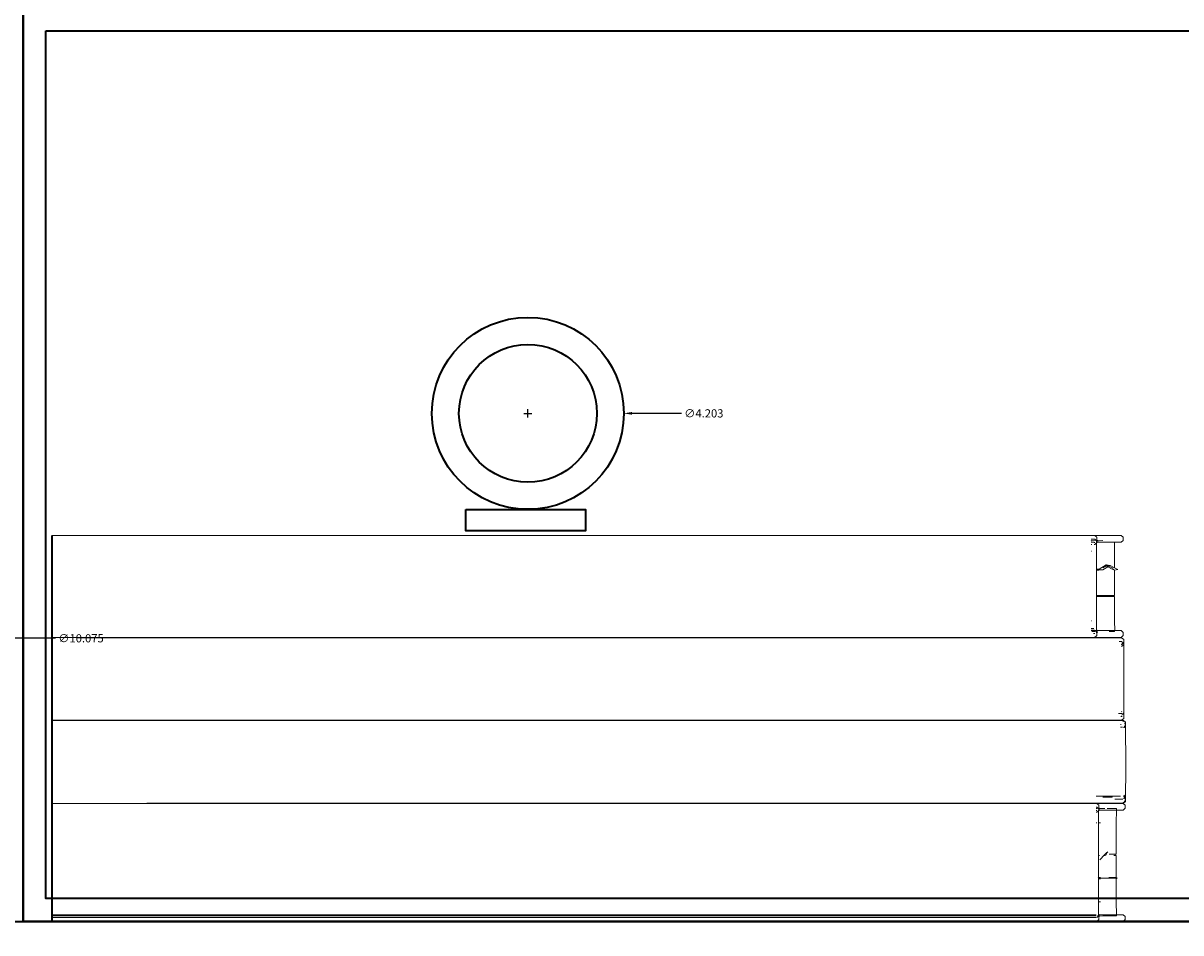
# Model space of a CAD drawing. Units: millimetres. Extents: x 446512 to 447461, y 70395 to 70610.
# Tile 17 of 39: x 446699 to 446725, y 70493 to 70513. Entities that reach past the tile are written whole.
import ezdxf

# ---------------------------------------------------------------- set-up
doc = ezdxf.new("R2010")
doc.units = ezdxf.units.MM
for name, color, linetype, lineweight in [('A-ANNO-DIMS', 2, 'Continuous', 18), ('A-FURN', 7, 'Continuous', 35), ('A-FURN-DECO', 8, 'Continuous', 13)]:
    doc.layers.add(name, color=color, linetype=linetype, lineweight=lineweight)
doc.styles.get("Standard").update_dxf_attribs({"font": 'arial.ttf'})
doc.dimstyles.get("Standard").update_dxf_attribs({"dimtxt": 0.18, "dimasz": 0.18, "dimexe": 0.18, "dimexo": 0.0625, "dimgap": 0.09, "dimtad": 0, "dimtih": 1, "dimtoh": 1, "dimdec": 4, "dimzin": 0, "dimdsep": 46, "dimtxsty": 'Standard', "dimcen": 0.09, "dimadec": 0, "dimazin": 0, "dimtfac": 1, "dimtdec": 4, "dimtofl": 0, "dimtmove": 0, "dimatfit": 3, "dimfxl": 1, "dimtolj": 1, "dimtzin": 0, "dimarcsym": 0})

# ---------------------------------------------------------------- blocks, each defined once
blk = doc.blocks.new('*D75')
at = {"layer": 'A-ANNO-DIMS', "color": 0, "lineweight": -2, "transparency": 16777216}
for p, q in [((446691.984, 70499.581), (446692.164, 70499.581)), ((446692.074, 70499.491), (446692.074, 70499.671)), ((446700.134, 70499.581), (446697.291, 70499.581))]:
    blk.add_line(p, q, dxfattribs=at)
at = {"layer": 'A-ANNO-DIMS', "color": 0, "transparency": 16777216}
blk.add_solid([(446697.291, 70499.611), (446697.291, 70499.551), (446697.111, 70499.581)], dxfattribs=at)
at = {"layer": 'Defpoints', "color": 0, "transparency": 16777216}
for p in [(446687.036, 70499.58), (446697.111, 70499.581)]:
    blk.add_point(p, dxfattribs=at)
at = {"layer": 'A-ANNO-DIMS', "color": 0, "transparency": 16777216, "insert": (446700.696, 70499.581), "char_height": 0.18, "attachment_point": 5}
blk.add_mtext('\\A1;∅10.075', dxfattribs=at)
blk = doc.blocks.new('*D77')
at = {"layer": 'A-ANNO-DIMS', "color": 0, "lineweight": -2, "transparency": 16777216}
for p, q in [((446710.394, 70504.505), (446710.574, 70504.505)), ((446710.484, 70504.415), (446710.484, 70504.595)), ((446713.847, 70504.505), (446712.766, 70504.505))]:
    blk.add_line(p, q, dxfattribs=at)
at = {"layer": 'A-ANNO-DIMS', "color": 0, "transparency": 16777216}
blk.add_solid([(446712.766, 70504.535), (446712.766, 70504.475), (446712.586, 70504.505)], dxfattribs=at)
at = {"layer": 'Defpoints', "color": 0, "transparency": 16777216}
for p in [(446708.383, 70504.506), (446712.586, 70504.505)]:
    blk.add_point(p, dxfattribs=at)
at = {"layer": 'A-ANNO-DIMS', "color": 0, "transparency": 16777216, "insert": (446714.338, 70504.505), "char_height": 0.18, "attachment_point": 5}
blk.add_mtext('\\A1;∅4.203', dxfattribs=at)

msp = doc.modelspace()

# ---------------------------------------------------------------- linework, layer by layer
at = {"layer": 'A-FURN'}
for p, q in [((446699.4288, 70513.3815), (446699.4288, 70493.3815)), ((446700.0643, 70493.3815), (446700.0643, 70501.8335)), ((446686.5728, 70493.3815), (446746.5728, 70493.3815))]:
    msp.add_line(p, q, dxfattribs=at)
for points in [[(446699.4288, 70513.3815), (446746.5728, 70513.3815), (446746.5728, 70493.3815), (446699.4288, 70493.3815)], [(446699.9288, 70512.8815), (446746.0728, 70512.8815), (446746.0728, 70493.8815), (446699.9288, 70493.8815)], [(446709.124, 70502.4015), (446711.7437, 70502.4015), (446711.7437, 70501.9339), (446709.124, 70501.9339)], [(446686.5728, 70493.3815), (446729.0084, 70493.3815), (446729.0084, 70473.3815), (446686.5728, 70473.3815)]]:
    msp.add_lwpolyline(points, close=True, dxfattribs=at)
for radius in [2.1014, 1.509]:
    msp.add_circle((446710.4845, 70504.5054), radius, dxfattribs=at)
at = {"layer": 'A-FURN-DECO'}
for p, q in [((446722.8971, 70501.8335), (446700.0643, 70501.8335)), ((446722.9157, 70501.8176), (446722.8971, 70501.8335)), ((446723.4803, 70501.8335), (446722.8971, 70501.8335)), ((446723.4803, 70501.8335), (446723.5262, 70501.7912)), ((446722.8352, 70501.6354), (446722.8233, 70501.6354)), ((446722.8288, 70501.7172), (446722.8234, 70501.7189)), ((446722.8234, 70501.6823), (446722.8913, 70501.6823)), ((446722.9054, 70501.7478), (446722.8235, 70501.7478)), ((446722.9205, 70501.7189), (446722.8288, 70501.7172)), ((446722.8982, 70501.676), (446722.8913, 70501.676)), ((446722.9054, 70501.6354), (446722.8913, 70501.6354)), ((446722.9015, 70501.6784), (446722.8982, 70501.676)), ((446722.9274, 70501.7275), (446722.9054, 70501.7478)), ((446722.9415, 70501.6688), (446722.9054, 70501.6354)), ((446722.9157, 70501.8176), (446722.9407, 70501.7992)), ((446722.9385, 70501.7172), (446722.9429, 70501.7175)), ((446722.943, 70501.713), (446722.9385, 70501.7172)), ((446722.9431, 70501.7102), (446722.9385, 70501.7067)), ((446722.9385, 70501.6823), (446722.9431, 70501.7102)), ((446722.9416, 70501.6777), (446722.9385, 70501.6823)), ((446722.9418, 70501.6823), (446722.9385, 70501.6823)), ((446722.9408, 70501.796), (446722.9407, 70501.7992)), ((446722.9435, 70501.7937), (446722.9408, 70501.796)), ((446722.941, 70501.4147), (446722.9413, 70501.6291)), ((446722.9413, 70501.6291), (446722.9415, 70501.6688)), ((446722.9512, 70501.6778), (446722.9415, 70501.6688)), ((446722.9415, 70501.6688), (446722.9416, 70501.6777)), ((446722.9525, 70501.6797), (446722.9418, 70501.6823)), ((446722.9429, 70501.7175), (446722.9461, 70501.7595)), ((446722.9429, 70501.7175), (446722.9499, 70501.7194)), ((446722.943, 70501.713), (446722.9429, 70501.7175)), ((446722.9512, 70501.7055), (446722.943, 70501.713)), ((446722.9431, 70501.7102), (446722.943, 70501.713)), ((446722.9461, 70501.7595), (446722.9435, 70501.7937)), ((446722.9499, 70501.7194), (446722.9461, 70501.7595)), ((446722.959, 70501.7246), (446722.9499, 70501.7194)), ((446722.9499, 70501.7194), (446722.9575, 70501.7183)), ((446722.9512, 70501.7055), (446722.9499, 70501.7194)), ((446722.9512, 70501.6778), (446722.9525, 70501.6797)), ((446722.9525, 70501.6797), (446722.9537, 70501.6907)), ((446722.9525, 70501.6797), (446722.9689, 70501.6823)), ((446722.9537, 70501.6907), (446722.9563, 70501.7131)), ((446722.9563, 70501.7131), (446722.9575, 70501.7183)), ((446722.9575, 70501.7183), (446722.959, 70501.7246)), ((446722.9575, 70501.7183), (446722.9672, 70501.7189)), ((446722.9689, 70501.6823), (446723.3347, 70501.6823)), ((446722.9919, 70501.7178), (446722.9821, 70501.7189)), ((446723.0764, 70501.7189), (446722.9919, 70501.7178)), ((446723.3347, 70501.6823), (446723.3328, 70501.4843)), ((446723.3347, 70501.6823), (446723.4803, 70501.6823)), ((446723.5262, 70501.7246), (446723.4803, 70501.6823)), ((446723.5262, 70501.7912), (446723.5262, 70501.7246)), ((446722.8269, 70501.4843), (446722.8232, 70501.4843)), ((446722.9383, 70501.0962), (446722.941, 70501.4147)), ((446723.3328, 70501.4843), (446723.3311, 70501.2268)), ((446722.9382, 70501.0737), (446722.9383, 70501.081)), ((446722.9382, 70501.0737), (446722.9408, 70501.0705)), ((446722.9382, 70501.0705), (446722.9382, 70501.0737)), ((446722.9408, 70501.0705), (446722.9382, 70501.0705)), ((446722.9407, 70500.9576), (446722.9382, 70501.0705)), ((446722.9408, 70501.0931), (446722.9383, 70501.0962)), ((446722.9383, 70501.0931), (446722.9383, 70501.0962)), ((446722.9383, 70501.0931), (446722.9408, 70501.0931)), ((446722.9383, 70501.0849), (446722.9383, 70501.0931)), ((446722.9383, 70501.0849), (446722.9408, 70501.0849)), ((446722.9383, 70501.081), (446722.9383, 70501.0849)), ((446722.9383, 70501.081), (446723.0064, 70501.0816)), ((446722.9845, 70501.0962), (446722.9408, 70501.0931)), ((446722.9408, 70501.0849), (446723.0064, 70501.0816)), ((446722.9879, 70501.0709), (446722.9408, 70501.0705)), ((446722.9845, 70501.0962), (446722.9879, 70501.0935)), ((446722.9879, 70501.0935), (446722.9926, 70501.0962)), ((446722.9927, 70501.0737), (446722.9879, 70501.0709)), ((446722.9962, 70501.0962), (446722.9926, 70501.0962)), ((446723.0795, 70501.0822), (446722.9927, 70501.0737)), ((446723.0064, 70501.0816), (446722.9927, 70501.0737)), ((446722.9962, 70501.0962), (446723.1508, 70501.1872)), ((446723.0064, 70501.0816), (446723.0093, 70501.0849)), ((446723.0795, 70501.0822), (446723.0093, 70501.0849)), ((446723.1507, 70501.1646), (446723.0776, 70501.1225)), ((446723.0795, 70501.0822), (446723.189, 70501.1452)), ((446723.1867, 70501.169), (446723.1507, 70501.1646)), ((446723.1729, 70501.1534), (446723.1507, 70501.1646)), ((446723.2423, 70501.1759), (446723.1508, 70501.1872)), ((446723.1508, 70501.1872), (446723.1867, 70501.169)), ((446723.2423, 70501.1759), (446723.1867, 70501.169)), ((446723.1867, 70501.169), (446723.2001, 70501.1622)), ((446723.189, 70501.1452), (446723.2099, 70501.1572)), ((446723.2861, 70501.0962), (446723.189, 70501.1452)), ((446723.2099, 70501.1572), (446723.2423, 70501.1759)), ((446723.2099, 70501.1572), (446723.296, 70501.1137)), ((446723.3308, 70501.126), (446723.2423, 70501.1759)), ((446723.3112, 70501.0962), (446723.2861, 70501.0962)), ((446723.3084, 70501.0849), (446723.2861, 70501.0962)), ((446723.3084, 70501.0849), (446723.3209, 70501.0849)), ((446723.3306, 70501.0737), (446723.3084, 70501.0849)), ((446723.3306, 70501.0737), (446723.3302, 70500.9431)), ((446723.4036, 70501.0849), (446723.3306, 70501.0737)), ((446723.3311, 70501.2268), (446723.3308, 70501.126)), ((446723.4036, 70501.0849), (446723.3308, 70501.126)), ((446722.9382, 70500.515), (446722.9407, 70500.9576)), ((446723.3302, 70500.515), (446723.3302, 70500.9431)), ((446722.9382, 70500.515), (446722.9875, 70500.5152)), ((446722.9382, 70500.4925), (446722.9382, 70500.515)), ((446722.9407, 70500.4471), (446722.9382, 70500.4925)), ((446722.9407, 70500.4925), (446722.9382, 70500.4925)), ((446722.9407, 70500.4925), (446722.9875, 70500.4926)), ((446722.9407, 70500.4471), (446722.9413, 70499.8035)), ((446722.9875, 70500.5152), (446723.3302, 70500.515)), ((446722.9875, 70500.4926), (446723.3303, 70500.4925)), ((446723.3302, 70500.515), (446723.1845, 70500.5038)), ((446723.1845, 70500.5038), (446723.3303, 70500.4925)), ((446723.3311, 70500.22), (446723.3303, 70500.4925)), ((446723.3311, 70500.22), (446723.3328, 70499.9625)), ((446722.8232, 70499.9625), (446722.8269, 70499.9625)), ((446722.9415, 70499.764), (446722.9413, 70499.8035)), ((446723.3328, 70499.9625), (446723.3382, 70499.7505)), ((446722.8971, 70499.5993), (446700.0643, 70499.5993)), ((446723.4896, 70499.5923), (446700.6021, 70499.5923)), ((446722.8794, 70499.7974), (446722.8233, 70499.7974)), ((446722.8924, 70499.7568), (446722.8234, 70499.7568)), ((446722.8234, 70499.7505), (446722.9065, 70499.7505)), ((446722.8402, 70499.7296), (446722.9199, 70499.7279)), ((446722.9199, 70499.7279), (446722.8415, 70499.7279)), ((446722.9002, 70499.685), (446722.876, 70499.685)), ((446722.8971, 70499.5993), (446722.9407, 70499.6336)), ((446722.8971, 70499.5993), (446723.4803, 70499.5993)), ((446722.9065, 70499.7505), (446722.9015, 70499.7543)), ((446722.9131, 70499.7505), (446722.9065, 70499.7505)), ((446722.9131, 70499.7505), (446722.9252, 70499.7394)), ((446722.9241, 70499.737), (446722.9131, 70499.7505)), ((446722.9303, 70499.7505), (446722.9131, 70499.7505)), ((446722.9415, 70499.764), (446722.9372, 70499.768)), ((446722.9385, 70499.7505), (446722.9416, 70499.7551)), ((446722.9418, 70499.7505), (446722.9385, 70499.7505)), ((446722.9385, 70499.7292), (446722.9385, 70499.7505)), ((446722.9385, 70499.7292), (446722.9429, 70499.7271)), ((446722.9429, 70499.7271), (446722.9385, 70499.727)), ((446722.943, 70499.7198), (446722.9385, 70499.7156)), ((446722.9407, 70499.6336), (446722.9436, 70499.6383)), ((446722.9416, 70499.7551), (446722.9415, 70499.764)), ((446722.9512, 70499.755), (446722.9415, 70499.764)), ((446722.9525, 70499.7531), (446722.9418, 70499.7505)), ((446722.9512, 70499.7273), (446722.9429, 70499.7271)), ((446722.9431, 70499.7225), (446722.9429, 70499.7271)), ((446722.9431, 70499.7225), (446722.943, 70499.7198)), ((446722.943, 70499.7198), (446722.9461, 70499.6702)), ((446722.943, 70499.7198), (446722.9499, 70499.7144)), ((446722.9512, 70499.7273), (446722.9431, 70499.7225)), ((446722.9436, 70499.6383), (446722.9461, 70499.6702)), ((446722.9461, 70499.6702), (446722.9499, 70499.7144)), ((446722.9499, 70499.7144), (446722.9512, 70499.7273)), ((446722.9499, 70499.7144), (446722.959, 70499.7081)), ((446722.9525, 70499.7531), (446722.9512, 70499.755)), ((446722.9689, 70499.7505), (446722.9525, 70499.7531)), ((446722.9538, 70499.7414), (446722.9525, 70499.7531)), ((446722.9563, 70499.7197), (446722.9538, 70499.7414)), ((446722.959, 70499.7081), (446722.9563, 70499.7197)), ((446723.3382, 70499.7505), (446722.9689, 70499.7505)), ((446723.2189, 70499.7283), (446723.2219, 70499.7279)), ((446723.335, 70499.7279), (446723.2219, 70499.7279)), ((446723.3382, 70499.7505), (446723.335, 70499.7279)), ((446723.3382, 70499.7505), (446723.4803, 70499.7505)), ((446723.4803, 70499.7505), (446723.5262, 70499.7081)), ((446723.5262, 70499.6416), (446723.4803, 70499.5993)), ((446723.4896, 70499.5923), (446723.5354, 70499.5511)), ((446723.5354, 70499.5535), (446723.4896, 70499.5923)), ((446723.4896, 70499.5923), (446723.5354, 70499.5589)), ((446723.5262, 70499.7081), (446723.5262, 70499.6416)), ((446723.5354, 70499.5535), (446723.5354, 70499.5589)), ((446723.5354, 70499.5511), (446723.5354, 70499.5535)), ((446723.5354, 70499.4881), (446723.5354, 70499.5511)), ((446723.4896, 70499.5089), (446723.437, 70499.5089)), ((446723.5241, 70499.4775), (446723.4896, 70499.5089)), ((446723.5241, 70499.4775), (446723.4896, 70499.4452)), ((446723.5327, 70499.4697), (446723.4896, 70499.439)), ((446723.5354, 70499.4407), (446723.4896, 70499.3996)), ((446723.5354, 70499.4881), (446723.5241, 70499.4775)), ((446723.5327, 70499.4697), (446723.5241, 70499.4775)), ((446723.5327, 70499.4697), (446723.5354, 70499.4751)), ((446723.5354, 70499.4717), (446723.5327, 70499.4697)), ((446723.5354, 70499.4673), (446723.5327, 70499.4697)), ((446723.5354, 70499.4751), (446723.5354, 70499.4881)), ((446723.5354, 70499.4751), (446723.5354, 70499.4717)), ((446723.5354, 70499.4717), (446723.5354, 70499.4673)), ((446723.5354, 70499.4695), (446723.5354, 70499.4717)), ((446723.5354, 70499.4673), (446723.5354, 70499.4695)), ((446723.5354, 70499.4407), (446723.5354, 70499.4673)), ((446723.5354, 70499.4407), (446723.5354, 70497.821)), ((446723.4896, 70497.7877), (446700.0643, 70497.7877)), ((446700.0643, 70497.7788), (446723.5109, 70497.7788)), ((446723.4216, 70497.9348), (446723.4896, 70497.9348)), ((446723.4896, 70497.871), (446723.4742, 70497.871)), ((446723.4971, 70497.9736), (446723.4896, 70497.9804)), ((446723.4896, 70497.9348), (446723.5163, 70497.9107)), ((446723.5042, 70497.8841), (446723.4896, 70497.871)), ((446723.5354, 70497.821), (446723.4896, 70497.7877)), ((446723.52, 70497.9188), (446723.4951, 70497.9369)), ((446723.5109, 70497.7788), (446723.5308, 70497.7608)), ((446723.5301, 70497.7788), (446723.5109, 70497.7788)), ((446723.5312, 70497.943), (446723.5252, 70497.9484)), ((446723.5301, 70497.7788), (446723.575, 70497.7454)), ((446723.4802, 70497.6954), (446723.4648, 70497.6954)), ((446723.5109, 70497.6317), (446723.4651, 70497.6317)), ((446723.5374, 70497.6299), (446723.5339, 70497.6313)), ((446723.5374, 70497.6299), (446723.5644, 70497.6542)), ((446723.5631, 70497.657), (446723.5561, 70497.6617)), ((446723.5574, 70497.7324), (446723.5593, 70497.7192)), ((446723.5644, 70497.6272), (446723.5583, 70497.6217)), ((446723.5593, 70497.7192), (446723.5605, 70497.6984)), ((446723.5623, 70497.6697), (446723.5631, 70497.657)), ((446723.5631, 70497.657), (446723.5644, 70497.6542)), ((446723.5644, 70497.6542), (446723.5694, 70497.6538)), ((446723.5658, 70497.6347), (446723.5644, 70497.6272)), ((446723.5694, 70497.6538), (446723.5658, 70497.6347)), ((446723.571, 70497.6582), (446723.5694, 70497.6538)), ((446723.571, 70497.6582), (446723.5732, 70497.684)), ((446723.5734, 70497.6912), (446723.575, 70497.7454)), ((446723.575, 70497.7454), (446723.5772, 70497.6891)), ((446723.5772, 70497.6891), (446723.5782, 70497.4065)), ((446723.5782, 70497.4065), (446723.5788, 70497.0652)), ((446723.5788, 70497.0652), (446723.5788, 70496.6735)), ((446723.5788, 70496.6735), (446723.5776, 70496.1388)), ((446723.2862, 70496.1212), (446722.9288, 70496.1212)), ((446723.2861, 70496.0998), (446723.0748, 70496.0988)), ((446723.2862, 70496.1212), (446723.2861, 70496.0998)), ((446723.4653, 70496.1212), (446723.2862, 70496.1212)), ((446723.5173, 70496.0575), (446723.3433, 70496.0575)), ((446723.575, 70496.0075), (446723.5301, 70495.9741)), ((446723.5631, 70496.0959), (446723.5328, 70496.0703)), ((446723.5644, 70496.0987), (446723.5329, 70496.1223)), ((446723.5644, 70496.1257), (446723.5385, 70496.149)), ((446723.5567, 70496.0153), (446723.5473, 70496.0069)), ((446723.5585, 70496.0282), (446723.5567, 70496.0153)), ((446723.5619, 70496.0757), (446723.5605, 70496.0545)), ((446723.5631, 70496.0959), (446723.5619, 70496.0757)), ((446723.5644, 70496.0987), (446723.5631, 70496.0959)), ((446723.5644, 70496.1257), (446723.5657, 70496.1183)), ((446723.5707, 70496.0978), (446723.5644, 70496.0987)), ((446723.5657, 70496.1183), (446723.5691, 70496.1025)), ((446723.5691, 70496.1025), (446723.5707, 70496.0978)), ((446723.5707, 70496.0978), (446723.5725, 70496.0941)), ((446723.5725, 70496.0941), (446723.5734, 70496.0617)), ((446723.5772, 70496.0638), (446723.5734, 70496.0617)), ((446723.575, 70496.0075), (446723.5734, 70496.0617)), ((446723.5776, 70496.1388), (446723.5772, 70496.0638)), ((446700.0643, 70495.9661), (446722.9411, 70495.9661)), ((446723.5301, 70495.9741), (446702.1377, 70495.9741)), ((446722.9493, 70495.7734), (446722.9349, 70495.7734)), ((446722.9422, 70495.8129), (446722.935, 70495.8129)), ((446722.9618, 70495.8516), (446722.9352, 70495.8515)), ((446722.9494, 70495.8828), (446722.9353, 70495.8828)), ((446722.9596, 70495.9506), (446722.9411, 70495.9661)), ((446722.9411, 70495.9661), (446723.5243, 70495.9661)), ((446722.9453, 70495.8152), (446722.9422, 70495.8129)), ((446722.9854, 70495.8059), (446722.9493, 70495.7734)), ((446722.9713, 70495.863), (446722.9494, 70495.8828)), ((446722.9825, 70495.9315), (446722.9596, 70495.9506)), ((446722.9596, 70495.9506), (446722.9846, 70495.9328)), ((446722.9816, 70495.5392), (446722.9851, 70495.7673)), ((446722.987, 70495.8462), (446722.9823, 70495.8427)), ((446722.9823, 70495.819), (446722.987, 70495.8462)), ((446722.9855, 70495.8145), (446722.9823, 70495.819)), ((446722.9857, 70495.819), (446722.9823, 70495.819)), ((446722.987, 70495.8489), (446722.9824, 70495.8531)), ((446722.9869, 70495.8531), (446722.9824, 70495.8531)), ((446722.9845, 70495.9298), (446722.9846, 70495.9328)), ((446722.9874, 70495.9274), (446722.9845, 70495.9298)), ((446722.9874, 70495.9274), (446722.9846, 70495.9328)), ((446722.9851, 70495.7673), (446722.9854, 70495.8059)), ((446722.9952, 70495.8146), (446722.9854, 70495.8059)), ((446722.9854, 70495.8059), (446722.9855, 70495.8145)), ((446722.9964, 70495.8165), (446722.9857, 70495.819)), ((446722.9869, 70495.8531), (446722.9901, 70495.8941)), ((446722.9938, 70495.8551), (446722.9869, 70495.8531)), ((446722.9869, 70495.8531), (446722.987, 70495.8489)), ((446722.9952, 70495.8416), (446722.987, 70495.8489)), ((446722.987, 70495.8462), (446722.987, 70495.8489)), ((446722.9901, 70495.8941), (446722.9874, 70495.9274)), ((446722.9938, 70495.8551), (446722.9901, 70495.8941)), ((446723.0029, 70495.8602), (446722.9938, 70495.8551)), ((446723.0012, 70495.8531), (446722.9938, 70495.8551)), ((446722.9952, 70495.8416), (446722.9938, 70495.8551)), ((446722.9952, 70495.8146), (446722.9964, 70495.8165)), ((446722.9964, 70495.8165), (446722.9976, 70495.8272)), ((446723.0807, 70495.819), (446722.9964, 70495.8165)), ((446722.9976, 70495.8272), (446723.0003, 70495.849)), ((446723.0003, 70495.849), (446723.0012, 70495.8531)), ((446723.0012, 70495.8531), (446723.0029, 70495.8602)), ((446723.0316, 70495.8518), (446723.0012, 70495.8531)), ((446723.1184, 70495.8529), (446723.0316, 70495.8518)), ((446723.3745, 70495.819), (446723.0807, 70495.819)), ((446723.1721, 70495.8529), (446723.1759, 70495.8523)), ((446723.3747, 70495.8529), (446723.1759, 70495.8523)), ((446723.3745, 70495.819), (446723.3725, 70495.5392)), ((446723.3747, 70495.8529), (446723.3745, 70495.819)), ((446723.3745, 70495.819), (446723.5243, 70495.819)), ((446723.5308, 70495.9921), (446723.5209, 70495.9832)), ((446723.5243, 70495.9661), (446723.5701, 70495.925)), ((446723.5701, 70495.8602), (446723.5243, 70495.819)), ((446723.5701, 70495.925), (446723.5701, 70495.8602)), ((446722.946, 70495.5392), (446722.9342, 70495.5392)), ((446722.9839, 70495.4518), (446722.9816, 70495.5392)), ((446723.0252, 70495.5392), (446722.9816, 70495.5392)), ((446723.3725, 70495.5392), (446723.3708, 70495.2072)), ((446722.9833, 70494.9427), (446722.9839, 70495.4518)), ((446723.37, 70494.8559), (446723.3708, 70495.2072)), ((446722.9808, 70494.8559), (446722.9833, 70494.9427)), ((446722.9808, 70494.8269), (446722.9808, 70494.8559)), ((446722.9808, 70494.8559), (446722.9914, 70494.8559)), ((446722.9833, 70494.3585), (446722.9808, 70494.8269)), ((446723.0026, 70494.8269), (446722.9808, 70494.8269)), ((446723.0114, 70494.7332), (446723.0272, 70494.7478)), ((446723.1026, 70494.8269), (446723.0272, 70494.7478)), ((446723.1026, 70494.8269), (446723.0924, 70494.8269)), ((446723.1372, 70494.8559), (446723.1026, 70494.8269)), ((446723.1026, 70494.8269), (446723.131, 70494.8559)), ((446723.138, 70494.8269), (446723.1139, 70494.8269)), ((446723.1221, 70494.8559), (446723.131, 70494.8559)), ((446723.131, 70494.8559), (446723.1663, 70494.8922)), ((446723.19, 70494.9068), (446723.1372, 70494.8559)), ((446723.1372, 70494.8559), (446723.1677, 70494.8559)), ((446723.1525, 70494.8269), (446723.1489, 70494.8269)), ((446723.19, 70494.9068), (446723.1663, 70494.8922)), ((446723.2167, 70494.8559), (446723.37, 70494.8559)), ((446723.3699, 70494.8269), (446723.3196, 70494.8269)), ((446723.37, 70494.8559), (446723.3383, 70494.8414)), ((446723.3383, 70494.8414), (446723.3699, 70494.8269)), ((446723.3699, 70494.5094), (446723.3699, 70494.8269)), ((446723.3699, 70494.5094), (446723.3703, 70494.341)), ((446722.9791, 70494.341), (446722.9833, 70494.3585)), ((446722.9808, 70494.3265), (446722.9791, 70494.341)), ((446723.0276, 70494.341), (446722.9791, 70494.341)), ((446722.9809, 70494.312), (446722.9808, 70494.3265)), ((446723.3909, 70494.3265), (446722.9808, 70494.3265)), ((446722.9839, 70493.8856), (446722.9809, 70494.312)), ((446722.9809, 70494.312), (446723.0242, 70494.312)), ((446723.3703, 70494.341), (446723.2129, 70494.341)), ((446723.3703, 70494.341), (446723.3909, 70494.3265)), ((446723.3704, 70494.312), (446723.3909, 70494.3265)), ((446723.3708, 70494.1436), (446723.3704, 70494.312)), ((446723.3708, 70494.1436), (446723.3725, 70493.8116)), ((446722.9816, 70493.8116), (446722.9839, 70493.8856)), ((446722.9851, 70493.5802), (446722.9816, 70493.8116)), ((446722.9816, 70493.8116), (446723.0251, 70493.8116)), ((446723.3725, 70493.8116), (446723.3746, 70493.5286)), ((446722.6925, 70493.5286), (446700.0643, 70493.5286)), ((446722.6925, 70493.5071), (446700.0643, 70493.5049)), ((446722.9353, 70493.4649), (446700.0643, 70493.4649)), ((446722.6925, 70493.5286), (446722.6925, 70493.5071)), ((446722.935, 70493.5286), (446722.6925, 70493.5286)), ((446722.6925, 70493.5071), (446722.8685, 70493.5066)), ((446722.8685, 70493.5066), (446722.9351, 70493.505)), ((446722.9494, 70493.4649), (446722.9441, 70493.4649)), ((446722.987, 70493.5015), (446722.9494, 70493.4649)), ((446722.9629, 70493.505), (446722.9834, 70493.505)), ((446722.9834, 70493.505), (446722.9679, 70493.5157)), ((446722.969, 70493.5179), (446722.9834, 70493.505)), ((446722.9857, 70493.5286), (446722.974, 70493.5286)), ((446722.9854, 70493.5418), (446722.9818, 70493.5451)), ((446722.9834, 70493.505), (446722.9857, 70493.5286)), ((446722.987, 70493.5015), (446722.9834, 70493.505)), ((446722.9854, 70493.5418), (446722.9851, 70493.5802)), ((446722.9855, 70493.5331), (446722.9854, 70493.5418)), ((446722.9952, 70493.5331), (446722.9854, 70493.5418)), ((446722.9857, 70493.5286), (446722.9855, 70493.5331)), ((446722.9964, 70493.5311), (446722.9857, 70493.5286)), ((446722.9952, 70493.5061), (446722.987, 70493.5015)), ((446722.987, 70493.5015), (446722.987, 70493.4988)), ((446722.987, 70493.5015), (446722.9939, 70493.4935)), ((446723.0003, 70493.4987), (446722.987, 70493.5015)), ((446722.987, 70493.4988), (446722.99, 70493.4506)), ((446722.99, 70493.4506), (446722.9939, 70493.4935)), ((446722.9939, 70493.4935), (446722.9952, 70493.5061)), ((446722.9939, 70493.4935), (446723.0029, 70493.4875)), ((446722.9964, 70493.5311), (446722.9952, 70493.5331)), ((446722.9952, 70493.5061), (446722.9995, 70493.505)), ((446723.0807, 70493.5286), (446722.9964, 70493.5311)), ((446722.9977, 70493.5199), (446722.9964, 70493.5311)), ((446722.9995, 70493.505), (446722.9977, 70493.5199)), ((446722.9995, 70493.505), (446723.0316, 70493.506)), ((446723.0003, 70493.4987), (446722.9995, 70493.505)), ((446723.1945, 70493.5055), (446723.0003, 70493.4987)), ((446723.0029, 70493.4875), (446723.0003, 70493.4987)), ((446723.0316, 70493.506), (446723.1945, 70493.5055)), ((446723.0807, 70493.5286), (446723.3746, 70493.5286)), ((446723.1945, 70493.5055), (446723.3747, 70493.505)), ((446723.3746, 70493.5286), (446723.3747, 70493.505)), ((446723.3746, 70493.5286), (446723.5243, 70493.5286)), ((446723.5243, 70493.5286), (446723.5701, 70493.4875)), ((446723.5701, 70493.4875), (446723.5701, 70493.4227)), ((446722.9411, 70493.3815), (446700.0643, 70493.3815)), ((446722.9411, 70493.3815), (446722.9846, 70493.4149)), ((446722.9411, 70493.3815), (446723.5243, 70493.3815)), ((446722.9846, 70493.4149), (446722.9875, 70493.4195)), ((446722.9875, 70493.4195), (446722.99, 70493.4506)), ((446723.5701, 70493.4227), (446723.5243, 70493.3815))]:
    msp.add_line(p, q, dxfattribs=at)

# ---------------------------------------------------------------- dimensions: what is measured, and where the dimension line sits
at = {"layer": 'A-ANNO-DIMS'}
for p1, p2, picture, middle in [((446708.3831, 70504.5059), (446712.5859, 70504.505), '*D77', (446713.8467, 70504.5047)), ((446687.0359, 70499.5805), (446697.1113, 70499.581), '*D75', (446700.134, 70499.5812))]:
    dim = msp.add_diameter_dim_2p(p1=p1, p2=p2, dimstyle='Standard', override={"dimdec": 3, "dimlfac": 1, "dimrnd": 0, "dimzin": 0, "dimdsep": 46, "dimlunit": 2}, dxfattribs=at)
    dim.commit()
    dim.dimension.update_dxf_attribs({"geometry": picture, "text_midpoint": middle, "dimtype": 163})

doc.saveas('drawing.dxf')
